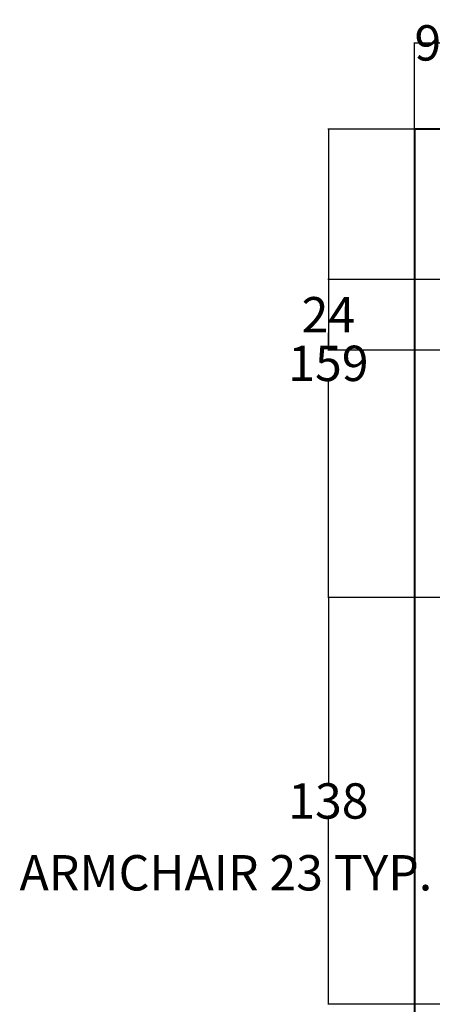
# Model space of a CAD drawing. Units: inches. Extents: x -124 to 612, y -69 to 524.
# Tile 2 of 9: x -124 to 16, y 190 to 524. Entities that reach past the tile are written whole.
import ezdxf

# ---------------------------------------------------------------- set-up
doc = ezdxf.new("R2010")
doc.units = ezdxf.units.IN
doc.header["$MEASUREMENT"] = 0
doc.layers.add('A-ANNO-DIMS', color=2, linetype='Continuous', lineweight=18)
doc.layers.add('A-WALL', color=7, linetype='Continuous', lineweight=40)
doc.styles.get("Standard").update_dxf_attribs({"font": 'arial.ttf'})
doc.dimstyles.get("Standard").update_dxf_attribs({"dimtxt": 12, "dimasz": 0.18, "dimexe": 0.18, "dimexo": 0.0625, "dimgap": 0.09, "dimtad": 0, "dimtih": 1, "dimtoh": 1, "dimdec": 0, "dimzin": 0, "dimdsep": 46, "dimlunit": 4, "dimtxsty": 'Standard', "dimcen": 0.09, "dimadec": 0, "dimazin": 0, "dimtfac": 1, "dimtdec": 0, "dimtofl": 0, "dimtmove": 0, "dimatfit": 3, "dimfxl": 1, "dimtolj": 1, "dimtzin": 0, "dimarcsym": 0})

# ---------------------------------------------------------------- blocks, each defined once
blk = doc.blocks.new('*D27')
at = {"layer": 'A-ANNO-DIMS', "color": 0, "lineweight": -2, "transparency": 16777216}
for p, q in [((23.16, 234.66), (22.98, 234.66)), ((23.16, 231.34), (23.16, 234.84)), ((45.48, 234.66), (23.34, 234.66)), ((45.66, 231.34), (45.66, 234.84))]:
    blk.add_line(p, q, dxfattribs=at)
at = {"layer": 'A-ANNO-DIMS', "color": 0, "transparency": 16777216}
for points in [[(23.34, 234.69), (23.34, 234.63), (23.16, 234.66)], [(45.48, 234.69), (45.48, 234.63), (45.66, 234.66)]]:
    blk.add_solid(points, dxfattribs=at)
at = {"layer": 'Defpoints', "color": 0, "transparency": 16777216}
for p in [(23.16, 234.66), (23.16, 231.28), (45.66, 231.28)]:
    blk.add_point(p, dxfattribs=at)
at = {"layer": 'A-ANNO-DIMS', "color": 0, "transparency": 16777216, "insert": (-53.7, 234.66), "char_height": 12, "attachment_point": 5}
blk.add_mtext('\\A1;ARMCHAIR 23 TYP.', dxfattribs=at)
blk = doc.blocks.new('*D47')
at = {"layer": 'A-ANNO-DIMS', "color": 0, "lineweight": -2, "transparency": 16777216}
for p, q in [((10.35, 487.09), (10.35, 516.46)), ((10.53, 516.28), (110.89, 516.28)), ((238.17, 516.28), (137.81, 516.28)), ((238.35, 487.09), (238.35, 516.46))]:
    blk.add_line(p, q, dxfattribs=at)
at = {"layer": 'A-ANNO-DIMS', "color": 0, "transparency": 16777216}
for points in [[(10.53, 516.31), (10.53, 516.25), (10.35, 516.28)], [(238.17, 516.31), (238.17, 516.25), (238.35, 516.28)]]:
    blk.add_solid(points, dxfattribs=at)
at = {"layer": 'Defpoints', "color": 0, "transparency": 16777216}
for p in [(238.35, 516.28), (10.35, 487.03), (238.35, 487.03)]:
    blk.add_point(p, dxfattribs=at)
at = {"layer": 'A-ANNO-DIMS', "color": 0, "transparency": 16777216, "insert": (124.35, 516.28), "char_height": 12, "attachment_point": 5}
blk.add_mtext('\\A1;228', dxfattribs=at)
blk = doc.blocks.new('*D53')
at = {"layer": 'A-ANNO-DIMS', "color": 0, "lineweight": -2, "transparency": 16777216}
for p, q in [((10.35, 487.09), (10.35, 516.46)), ((10.53, 516.28), (10.82, 516.28)), ((19.17, 516.28), (18.89, 516.28)), ((19.35, 478.09), (19.35, 516.46))]:
    blk.add_line(p, q, dxfattribs=at)
at = {"layer": 'A-ANNO-DIMS', "color": 0, "transparency": 16777216}
for points in [[(10.53, 516.31), (10.53, 516.25), (10.35, 516.28)], [(19.17, 516.31), (19.17, 516.25), (19.35, 516.28)]]:
    blk.add_solid(points, dxfattribs=at)
at = {"layer": 'Defpoints', "color": 0, "transparency": 16777216}
for p in [(10.35, 516.28), (10.35, 487.03), (19.35, 478.03)]:
    blk.add_point(p, dxfattribs=at)
at = {"layer": 'A-ANNO-DIMS', "color": 0, "transparency": 16777216, "insert": (14.85, 516.28), "char_height": 12, "attachment_point": 5}
blk.add_mtext('\\A1;9', dxfattribs=at)
blk = doc.blocks.new('*D56')
at = {"layer": 'A-ANNO-DIMS', "color": 0, "lineweight": -2, "transparency": 16777216}
for p, q in [((19.29, 328.03), (-19.08, 328.03)), ((-18.9, 327.85), (-18.9, 265.25)), ((-18.9, 190.21), (-18.9, 252.81)), ((19.29, 190.03), (-19.08, 190.03))]:
    blk.add_line(p, q, dxfattribs=at)
at = {"layer": 'A-ANNO-DIMS', "color": 0, "transparency": 16777216}
for points in [[(-18.93, 327.85), (-18.87, 327.85), (-18.9, 328.03)], [(-18.93, 190.21), (-18.87, 190.21), (-18.9, 190.03)]]:
    blk.add_solid(points, dxfattribs=at)
at = {"layer": 'Defpoints', "color": 0, "transparency": 16777216}
for p in [(-18.9, 328.03), (19.35, 328.03), (19.35, 190.03)]:
    blk.add_point(p, dxfattribs=at)
at = {"layer": 'A-ANNO-DIMS', "color": 0, "transparency": 16777216, "insert": (-18.9, 259.03), "char_height": 12, "attachment_point": 5}
blk.add_mtext('\\A1;138', dxfattribs=at)
blk = doc.blocks.new('*D57')
at = {"layer": 'A-ANNO-DIMS', "color": 0, "lineweight": -2, "transparency": 16777216}
for p, q in [((10.29, 487.03), (-19.08, 487.03)), ((-18.9, 486.85), (-18.9, 413.75)), ((-18.9, 328.21), (-18.9, 401.31)), ((19.29, 328.03), (-19.08, 328.03))]:
    blk.add_line(p, q, dxfattribs=at)
at = {"layer": 'A-ANNO-DIMS', "color": 0, "transparency": 16777216}
for points in [[(-18.93, 486.85), (-18.87, 486.85), (-18.9, 487.03)], [(-18.93, 328.21), (-18.87, 328.21), (-18.9, 328.03)]]:
    blk.add_solid(points, dxfattribs=at)
at = {"layer": 'Defpoints', "color": 0, "transparency": 16777216}
for p in [(-18.9, 487.03), (10.35, 487.03), (19.35, 328.03)]:
    blk.add_point(p, dxfattribs=at)
at = {"layer": 'A-ANNO-DIMS', "color": 0, "transparency": 16777216, "insert": (-18.9, 407.53), "char_height": 12, "attachment_point": 5}
blk.add_mtext('\\A1;159', dxfattribs=at)
blk = doc.blocks.new('*D71')
at = {"layer": 'A-ANNO-DIMS', "color": 0, "lineweight": -2, "transparency": 16777216}
for p, q in [((158.29, 436.03), (-19.08, 436.03)), ((-18.9, 435.85), (-18.9, 430.14)), ((-18.9, 412.21), (-18.9, 417.91)), ((158.29, 412.03), (-19.08, 412.03))]:
    blk.add_line(p, q, dxfattribs=at)
at = {"layer": 'A-ANNO-DIMS', "color": 0, "transparency": 16777216}
for points in [[(-18.93, 435.85), (-18.87, 435.85), (-18.9, 436.03)], [(-18.93, 412.21), (-18.87, 412.21), (-18.9, 412.03)]]:
    blk.add_solid(points, dxfattribs=at)
at = {"layer": 'Defpoints', "color": 0, "transparency": 16777216}
for p in [(-18.9, 436.03), (158.35, 436.03), (158.35, 412.03)]:
    blk.add_point(p, dxfattribs=at)
at = {"layer": 'A-ANNO-DIMS', "color": 0, "transparency": 16777216, "insert": (-18.9, 424.03), "char_height": 12, "attachment_point": 5}
blk.add_mtext('\\A1;24', dxfattribs=at)

msp = doc.modelspace()

# ---------------------------------------------------------------- linework, layer by layer
at = {"layer": 'A-WALL'}
msp.add_lwpolyline([(10.3513, 7.0291), (238.3513, 7.0291), (238.3513, 487.0291), (10.3513, 487.0291)], close=True, dxfattribs=at)

# ---------------------------------------------------------------- dimensions: what is measured, and where the dimension line sits
at = {"layer": 'A-ANNO-DIMS'}
for base, p1, p2, picture, middle in [((10.3513, 516.2791), (19.3513, 478.0291), (10.3513, 487.0291), '*D53', (14.8513, 516.2791)), ((238.3513, 516.2791), (10.3513, 487.0291), (238.3513, 487.0291), '*D47', (124.3513, 516.2791))]:
    dim = msp.add_linear_dim(base=base, p1=p1, p2=p2, dimstyle='Standard', override={"dimdec": 0, "dimlfac": 1, "dimrnd": 0, "dimzin": 0, "dimdsep": 46, "dimlunit": 2}, dxfattribs=at)
    dim.commit()
    dim.dimension.update_dxf_attribs({"geometry": picture, "text_midpoint": middle})
for base, p1, p2, picture, middle in [((-18.8987, 487.0291), (19.3513, 328.0291), (10.3513, 487.0291), '*D57', (-18.8987, 407.5291)), ((-18.8987, 436.0291), (158.3513, 412.0291), (158.3513, 436.0291), '*D71', (-18.8987, 424.0291)), ((-18.8987, 328.0291), (19.3513, 190.0291), (19.3513, 328.0291), '*D56', (-18.8987, 259.0291))]:
    dim = msp.add_linear_dim(base=base, p1=p1, p2=p2, angle=90, dimstyle='Standard', override={"dimdec": 0, "dimlfac": 1, "dimrnd": 0, "dimzin": 0, "dimdsep": 46, "dimlunit": 2}, dxfattribs=at)
    dim.commit()
    dim.dimension.update_dxf_attribs({"geometry": picture, "text_midpoint": middle})
dim = msp.add_linear_dim(base=(23.1554, 234.656), p1=(45.6588, 231.2805), p2=(23.1554, 231.2805), angle=180, text='ARMCHAIR <> TYP.', dimstyle='Standard', override={"dimdec": 0, "dimlfac": 1, "dimrnd": 0, "dimzin": 0, "dimdsep": 46, "dimlunit": 2}, dxfattribs=at)
dim.commit()
dim.dimension.update_dxf_attribs({"geometry": '*D27', "text_midpoint": (-53.7026, 234.656)})

doc.saveas('drawing.dxf')
